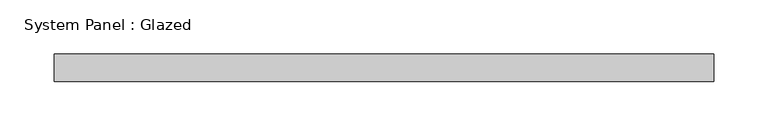
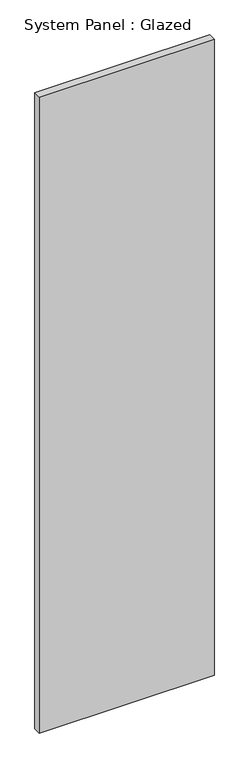
"""IFC4 building model written with IfcOpenShell, lengths in millimetres: plate geometry, System Panel : Glazed."""

from ifc_helpers import new_model, si_unit, origin, origin_with_axes, place, context, project, spatial, polyline, outline, extrude, source, transform, mapped, element, save


def system_panel_glazed_bc4b8a1a(model_context):
    return source(origin(), model_context, "Body", "SweptSolid", [
        extrude(outline(polyline([(304.8, 19.05), (-304.8, 19.05), (-304.8, 44.45), (304.8, 44.45), (304.8, 19.05)])), origin_with_axes(), (0.0, 0.0, 1.0), 2343.15),
    ])


if __name__ == "__main__":
    model = new_model("IFC4")
    model_context = context("Model", 3, world=origin())
    ifc_project = project(units=[si_unit("LENGTHUNIT", "METRE", prefix="MILLI")], contexts=[model_context])
    site = spatial("IfcSite", under=ifc_project)
    building = spatial("IfcBuilding", under=site)
    placement = place(None, origin())
    system_panel_glazed_shape = system_panel_glazed_bc4b8a1a(model_context)
    element("IfcPlate", 1, ObjectType="System Panel : Glazed", at=placement, inside=building, context=model_context, shape_type="MappedRepresentation", body=[
        mapped(system_panel_glazed_shape, transform((0.0, 0.0, 0.0), x_axis=(1.0, 0.0, 0.0), y_axis=(0.0, 1.0, 0.0), z_axis=(0.0, 0.0, 1.0))),
    ])
    save(model, "model.ifc")

# Revit data of these elements
# Type "System Panel : Glazed"
#   Construction Type Id = "GSP4R"
#   Analytic Construction = "1/8 in Pilkington single glazing"
#   Visual Light Transmittance = 0.9
#   Solar Heat Gain Coefficient = 0.86
#   Heat Transfer Coefficient (U) = 1.18115 BTU/(h·ft²·°F)
#   Define Thermal Properties by = 1
# Element 1 (IfcPlate, "System Panel : Glazed")
#   Materials on its faces: "Glass"
# Materials
#   "Glass": class "Glass", colour RGB 0 128 192, transparency 0.75, Description = "Soda Lime Glass", Cost = 0
